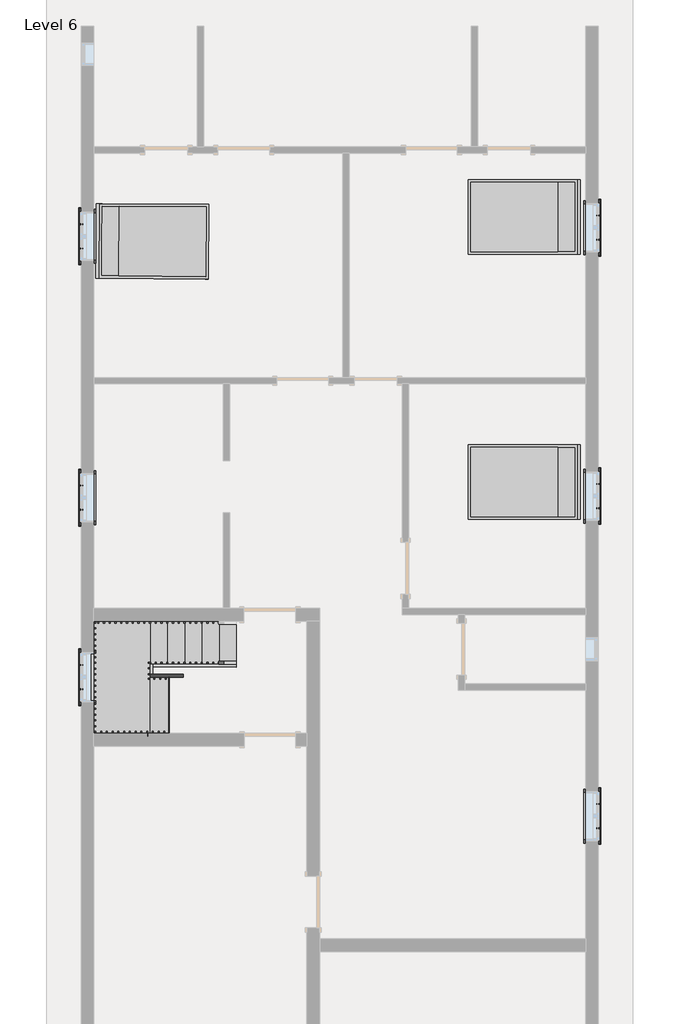
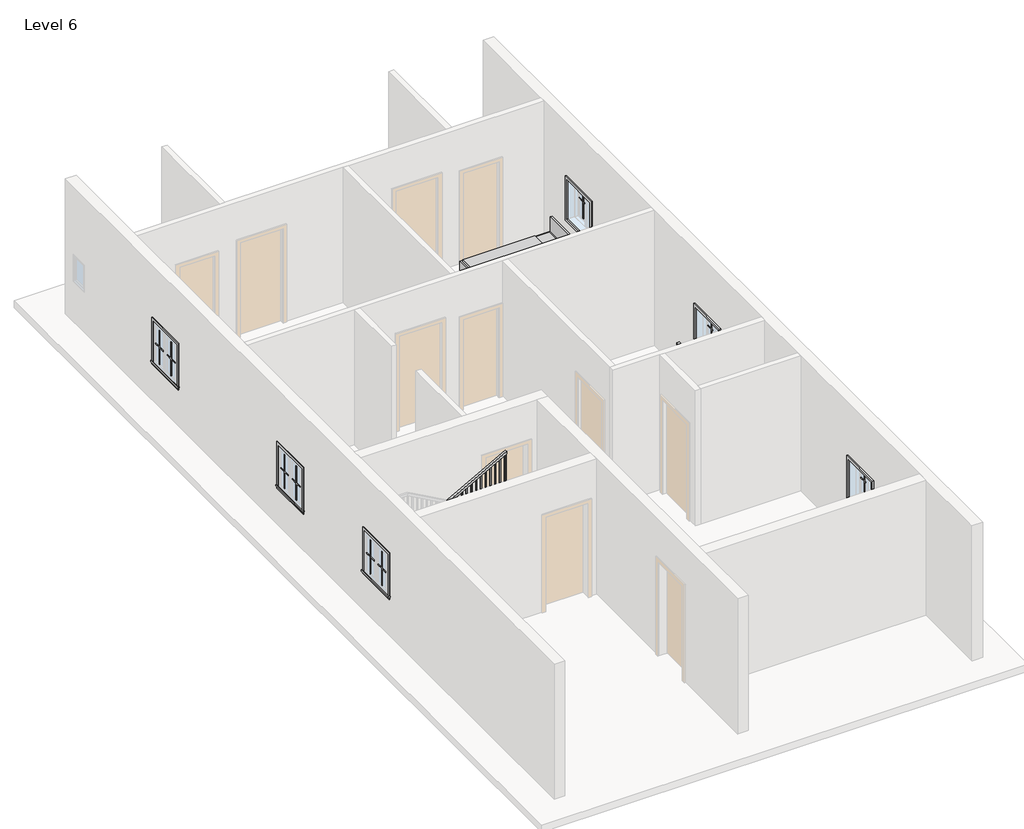
# One storey, part 3 of 3: 24 proxies, 6 members, 3 furniture elements, 1 railing, 1 stair flight.
"""IFC4 building model written with IfcOpenShell, lengths in millimetres."""

from ifc_helpers import new_model, si_unit, frame, origin, place, context, project, spatial, polyline, outline, extrude, faceted_brep, transform, mapped, element, save
from components import muntin_pattern_2x2_muntin_pattern_2x2_b3fe6957, muntin_pattern_2x2_muntin_pattern_2x2_3e0ecaf2, trim_window_exterior_flat_with_sill_41619996, trim_window_interior_flat_picture_frame_51c85655, bed_17739_bed_17739_15c61121, stair_flight_ed5f4c0f

model = new_model("IFC4")

# Units and contexts
model_context = context("Model", 3, world=origin())
ifc_project = project(units=[si_unit("LENGTHUNIT", "METRE", prefix="MILLI")], contexts=[model_context])

# Site, building, storey
site = spatial("IfcSite", under=ifc_project)
building = spatial("IfcBuilding", under=site)
storey = spatial("IfcBuildingStorey", under=building, Name="Level 6", Elevation=12801.6)

# Proxies
placement = place(None, origin())
muntin_pattern_2x2_muntin_pattern_2x2_shape = muntin_pattern_2x2_muntin_pattern_2x2_b3fe6957(model_context)
element("IfcBuildingElementProxy", 1, Name="Muntin Pattern_2x2 : Muntin Pattern_2x2", ObjectType="Muntin Pattern_2x2 : Muntin Pattern_2x2", at=placement, inside=storey, context=model_context, shape_type="MappedRepresentation", body=[
    mapped(muntin_pattern_2x2_muntin_pattern_2x2_shape, transform((3307.2334916, 6850.4197267, 13785.85), x_axis=(0.0, -1.0, 0.0), y_axis=(1.0, 0.0, 0.0), z_axis=(0.0, 0.0, 1.0))),
])
element("IfcBuildingElementProxy", 2, Name="Muntin Pattern_2x2 : Muntin Pattern_2x2", ObjectType="Muntin Pattern_2x2 : Muntin Pattern_2x2", at=placement, inside=storey, context=model_context, shape_type="MappedRepresentation", body=[
    mapped(muntin_pattern_2x2_muntin_pattern_2x2_shape, transform((3307.2334916, 2106.9697267, 13785.85), x_axis=(0.0, -1.0, 0.0), y_axis=(1.0, 0.0, 0.0), z_axis=(0.0, 0.0, 1.0))),
])
element("IfcBuildingElementProxy", 3, Name="Muntin Pattern_2x2 : Muntin Pattern_2x2", ObjectType="Muntin Pattern_2x2 : Muntin Pattern_2x2", at=placement, inside=storey, context=model_context, shape_type="MappedRepresentation", body=[
    mapped(muntin_pattern_2x2_muntin_pattern_2x2_shape, transform((-5817.7165084, 6269.3947267, 13785.85), x_axis=(0.0, 1.0, 0.0), y_axis=(-1.0, 0.0, 0.0), z_axis=(0.0, 0.0, 1.0))),
])
element("IfcBuildingElementProxy", 4, Name="Muntin Pattern_2x2 : Muntin Pattern_2x2", ObjectType="Muntin Pattern_2x2 : Muntin Pattern_2x2", at=placement, inside=storey, context=model_context, shape_type="MappedRepresentation", body=[
    mapped(muntin_pattern_2x2_muntin_pattern_2x2_shape, transform((-5817.7165084, 1649.7697267, 13785.85), x_axis=(0.0, 1.0, 0.0), y_axis=(-1.0, 0.0, 0.0), z_axis=(0.0, 0.0, 1.0))),
])
element("IfcBuildingElementProxy", 5, Name="Muntin Pattern_2x2 : Muntin Pattern_2x2", ObjectType="Muntin Pattern_2x2 : Muntin Pattern_2x2", at=placement, inside=storey, context=model_context, shape_type="MappedRepresentation", body=[
    mapped(muntin_pattern_2x2_muntin_pattern_2x2_shape, transform((3307.2334916, -3547.7052733, 13785.85), x_axis=(0.0, -1.0, 0.0), y_axis=(1.0, 0.0, 0.0), z_axis=(0.0, 0.0, 1.0))),
])
element("IfcBuildingElementProxy", 6, Name="Muntin Pattern_2x2 : Muntin Pattern_2x2", ObjectType="Muntin Pattern_2x2 : Muntin Pattern_2x2", at=placement, inside=storey, context=model_context, shape_type="MappedRepresentation", body=[
    mapped(muntin_pattern_2x2_muntin_pattern_2x2_shape, transform((-5817.7165084, -1522.0552733, 13785.85), x_axis=(0.0, 1.0, 0.0), y_axis=(-1.0, 0.0, 0.0), z_axis=(0.0, 0.0, 1.0))),
])
muntin_pattern_2x2_muntin_pattern_2x2_2_shape = muntin_pattern_2x2_muntin_pattern_2x2_3e0ecaf2(model_context)
element("IfcBuildingElementProxy", 7, Name="Muntin Pattern_2x2 : Muntin Pattern_2x2", ObjectType="Muntin Pattern_2x2 : Muntin Pattern_2x2", at=placement, inside=storey, context=model_context, shape_type="MappedRepresentation", body=[
    mapped(muntin_pattern_2x2_muntin_pattern_2x2_2_shape, transform((3307.2334916, 6421.7947267, 13785.85), x_axis=(0.0, 1.0, 0.0), y_axis=(-1.0, 0.0, 0.0), z_axis=(0.0, 0.0, 1.0))),
])
element("IfcBuildingElementProxy", 8, Name="Muntin Pattern_2x2 : Muntin Pattern_2x2", ObjectType="Muntin Pattern_2x2 : Muntin Pattern_2x2", at=placement, inside=storey, context=model_context, shape_type="MappedRepresentation", body=[
    mapped(muntin_pattern_2x2_muntin_pattern_2x2_2_shape, transform((3307.2334916, 1678.3447267, 13785.85), x_axis=(0.0, 1.0, 0.0), y_axis=(-1.0, 0.0, 0.0), z_axis=(0.0, 0.0, 1.0))),
])
element("IfcBuildingElementProxy", 9, Name="Muntin Pattern_2x2 : Muntin Pattern_2x2", ObjectType="Muntin Pattern_2x2 : Muntin Pattern_2x2", at=placement, inside=storey, context=model_context, shape_type="MappedRepresentation", body=[
    mapped(muntin_pattern_2x2_muntin_pattern_2x2_2_shape, transform((-5817.7165084, 6698.0197267, 13785.85), x_axis=(0.0, -1.0, 0.0), y_axis=(1.0, 0.0, 0.0), z_axis=(0.0, 0.0, 1.0))),
])
element("IfcBuildingElementProxy", 10, Name="Muntin Pattern_2x2 : Muntin Pattern_2x2", ObjectType="Muntin Pattern_2x2 : Muntin Pattern_2x2", at=placement, inside=storey, context=model_context, shape_type="MappedRepresentation", body=[
    mapped(muntin_pattern_2x2_muntin_pattern_2x2_2_shape, transform((-5817.7165084, 2078.3947267, 13785.85), x_axis=(0.0, -1.0, 0.0), y_axis=(1.0, 0.0, 0.0), z_axis=(0.0, 0.0, 1.0))),
])
element("IfcBuildingElementProxy", 11, Name="Muntin Pattern_2x2 : Muntin Pattern_2x2", ObjectType="Muntin Pattern_2x2 : Muntin Pattern_2x2", at=placement, inside=storey, context=model_context, shape_type="MappedRepresentation", body=[
    mapped(muntin_pattern_2x2_muntin_pattern_2x2_2_shape, transform((3307.2334916, -3976.3302733, 13785.85), x_axis=(0.0, 1.0, 0.0), y_axis=(-1.0, 0.0, 0.0), z_axis=(0.0, 0.0, 1.0))),
])
element("IfcBuildingElementProxy", 12, Name="Muntin Pattern_2x2 : Muntin Pattern_2x2", ObjectType="Muntin Pattern_2x2 : Muntin Pattern_2x2", at=placement, inside=storey, context=model_context, shape_type="MappedRepresentation", body=[
    mapped(muntin_pattern_2x2_muntin_pattern_2x2_2_shape, transform((-5817.7165084, -1093.4302733, 13785.85), x_axis=(0.0, -1.0, 0.0), y_axis=(1.0, 0.0, 0.0), z_axis=(0.0, 0.0, 1.0))),
])
trim_window_exterior_flat_with_sill_shape = trim_window_exterior_flat_with_sill_41619996(model_context)
element("IfcBuildingElementProxy", 13, Name="Trim-Window-Exterior-Flat : with Sill", ObjectType="Trim-Window-Exterior-Flat : with Sill", at=placement, inside=storey, context=model_context, shape_type="MappedRepresentation", body=[
    mapped(trim_window_exterior_flat_with_sill_shape, transform((3316.7584916, 6636.1072267, 14630.4), x_axis=(0.0, 1.0, 0.0), y_axis=(0.0, 0.0, 1.0), z_axis=(1.0, 0.0, 0.0))),
])
element("IfcBuildingElementProxy", 14, Name="Trim-Window-Exterior-Flat : with Sill", ObjectType="Trim-Window-Exterior-Flat : with Sill", at=placement, inside=storey, context=model_context, shape_type="MappedRepresentation", body=[
    mapped(trim_window_exterior_flat_with_sill_shape, transform((3316.7584916, 1892.6572267, 14630.4), x_axis=(0.0, 1.0, 0.0), y_axis=(0.0, 0.0, 1.0), z_axis=(1.0, 0.0, 0.0))),
])
element("IfcBuildingElementProxy", 15, Name="Trim-Window-Exterior-Flat : with Sill", ObjectType="Trim-Window-Exterior-Flat : with Sill", at=placement, inside=storey, context=model_context, shape_type="MappedRepresentation", body=[
    mapped(trim_window_exterior_flat_with_sill_shape, transform((-5827.2415084, 6483.7072267, 14630.4), x_axis=(0.0, -1.0, 0.0), y_axis=(0.0, 0.0, 1.0), z_axis=(-1.0, 0.0, 0.0))),
])
element("IfcBuildingElementProxy", 16, Name="Trim-Window-Exterior-Flat : with Sill", ObjectType="Trim-Window-Exterior-Flat : with Sill", at=placement, inside=storey, context=model_context, shape_type="MappedRepresentation", body=[
    mapped(trim_window_exterior_flat_with_sill_shape, transform((-5827.2415084, 1864.0822267, 14630.4), x_axis=(0.0, -1.0, 0.0), y_axis=(0.0, 0.0, 1.0), z_axis=(-1.0, 0.0, 0.0))),
])
element("IfcBuildingElementProxy", 17, Name="Trim-Window-Exterior-Flat : with Sill", ObjectType="Trim-Window-Exterior-Flat : with Sill", at=placement, inside=storey, context=model_context, shape_type="MappedRepresentation", body=[
    mapped(trim_window_exterior_flat_with_sill_shape, transform((3316.7584916, -3762.0177733, 14630.4), x_axis=(0.0, 1.0, 0.0), y_axis=(0.0, 0.0, 1.0), z_axis=(1.0, 0.0, 0.0))),
])
element("IfcBuildingElementProxy", 18, Name="Trim-Window-Exterior-Flat : with Sill", ObjectType="Trim-Window-Exterior-Flat : with Sill", at=placement, inside=storey, context=model_context, shape_type="MappedRepresentation", body=[
    mapped(trim_window_exterior_flat_with_sill_shape, transform((-5827.2415084, -1307.7427733, 14630.4), x_axis=(0.0, -1.0, 0.0), y_axis=(0.0, 0.0, 1.0), z_axis=(-1.0, 0.0, 0.0))),
])
trim_window_interior_flat_picture_frame_shape = trim_window_interior_flat_picture_frame_51c85655(model_context)
element("IfcBuildingElementProxy", 19, Name="Trim-Window-Interior-Flat : Picture Frame", ObjectType="Trim-Window-Interior-Flat : Picture Frame", at=placement, inside=storey, context=model_context, shape_type="MappedRepresentation", body=[
    mapped(trim_window_interior_flat_picture_frame_shape, transform((3088.1584916, 6636.1072267, 14630.4), x_axis=(0.0, -1.0, 0.0), y_axis=(0.0, 0.0, 1.0), z_axis=(-1.0, 0.0, 0.0))),
])
element("IfcBuildingElementProxy", 20, Name="Trim-Window-Interior-Flat : Picture Frame", ObjectType="Trim-Window-Interior-Flat : Picture Frame", at=placement, inside=storey, context=model_context, shape_type="MappedRepresentation", body=[
    mapped(trim_window_interior_flat_picture_frame_shape, transform((3088.1584916, 1892.6572267, 14630.4), x_axis=(0.0, -1.0, 0.0), y_axis=(0.0, 0.0, 1.0), z_axis=(-1.0, 0.0, 0.0))),
])
element("IfcBuildingElementProxy", 21, Name="Trim-Window-Interior-Flat : Picture Frame", ObjectType="Trim-Window-Interior-Flat : Picture Frame", at=placement, inside=storey, context=model_context, shape_type="MappedRepresentation", body=[
    mapped(trim_window_interior_flat_picture_frame_shape, transform((-5598.6415084, 6483.7072267, 14630.4), x_axis=(0.0, 1.0, 0.0), y_axis=(0.0, 0.0, 1.0), z_axis=(1.0, 0.0, 0.0))),
])
element("IfcBuildingElementProxy", 22, Name="Trim-Window-Interior-Flat : Picture Frame", ObjectType="Trim-Window-Interior-Flat : Picture Frame", at=placement, inside=storey, context=model_context, shape_type="MappedRepresentation", body=[
    mapped(trim_window_interior_flat_picture_frame_shape, transform((-5598.6415084, 1864.0822267, 14630.4), x_axis=(0.0, 1.0, 0.0), y_axis=(0.0, 0.0, 1.0), z_axis=(1.0, 0.0, 0.0))),
])
element("IfcBuildingElementProxy", 23, Name="Trim-Window-Interior-Flat : Picture Frame", ObjectType="Trim-Window-Interior-Flat : Picture Frame", at=placement, inside=storey, context=model_context, shape_type="MappedRepresentation", body=[
    mapped(trim_window_interior_flat_picture_frame_shape, transform((3088.1584916, -3762.0177733, 14630.4), x_axis=(0.0, -1.0, 0.0), y_axis=(0.0, 0.0, 1.0), z_axis=(-1.0, 0.0, 0.0))),
])
element("IfcBuildingElementProxy", 24, Name="Trim-Window-Interior-Flat : Picture Frame", ObjectType="Trim-Window-Interior-Flat : Picture Frame", at=placement, inside=storey, context=model_context, shape_type="MappedRepresentation", body=[
    mapped(trim_window_interior_flat_picture_frame_shape, transform((-5598.6415084, -1307.7427733, 14630.4), x_axis=(0.0, 1.0, 0.0), y_axis=(0.0, 0.0, 1.0), z_axis=(1.0, 0.0, 0.0))),
])

# Furniture
bed_17739_bed_17739_shape = bed_17739_bed_17739_15c61121(model_context)
element("IfcFurniture", 25, ObjectType="Bed_17739 : Bed_17739", at=placement, inside=storey, context=model_context, shape_type="MappedRepresentation", body=[
    mapped(bed_17739_bed_17739_shape, transform((-4543.6279345, 6394.2844586, 12801.6), x_axis=(0.007593038844487308, 0.9999711724650396, 0.0), y_axis=(-0.9999711724650396, 0.007593038844487308, 0.0), z_axis=(0.0, 0.0, 1.0))),
])
element("IfcFurniture", 26, ObjectType="Bed_17739 : Bed_17739", at=placement, inside=storey, context=model_context, shape_type="MappedRepresentation", body=[
    mapped(bed_17739_bed_17739_shape, transform((1983.2584916, 6826.6072267, 12801.6), x_axis=(0.0, -1.0, 0.0), y_axis=(1.0, 0.0, 0.0), z_axis=(0.0, 0.0, 1.0))),
])
element("IfcFurniture", 27, ObjectType="Bed_17739 : Bed_17739", at=placement, inside=storey, context=model_context, shape_type="MappedRepresentation", body=[
    mapped(bed_17739_bed_17739_shape, transform((1983.2584916, 2140.3072267, 12801.6), x_axis=(0.0, -1.0, 0.0), y_axis=(1.0, 0.0, 0.0), z_axis=(0.0, 0.0, 1.0))),
])

# Members
element("IfcMember", 28, ObjectType="Stringer - 2\" Width", at=placement, inside=storey, context=model_context, shape_type="SweptSolid", body=[
    extrude(outline(polyline([(12801.6, -3084.0415084), (13009.1983948, -3084.0415084), (13827.6428392, -4557.2415084), (13478.9641651, -4557.2415084), (12801.6, -3337.9860112), (12801.6, -3084.0415084)])), frame((0.0, -1127.4758739, 0.0), z_axis=(0.0, 1.0, 0.0), x_axis=(0.0, 0.0, 1.0)), (0.0, 0.0, 1.0), 50.8),
])
element("IfcMember", 29, ObjectType="Stringer - 2\" Width", at=placement, inside=storey, context=model_context, shape_type="SweptSolid", body=[
    extrude(outline(polyline([(-4608.0415084, -1076.6758739), (-4557.2415084, -1076.6758739), (-4557.2415084, -1256.9427733), (-4608.0415084, -1256.9427733), (-4608.0415084, -1076.6758739)])), frame((0.0, 0.0, 13589.0), z_axis=(0.0, 0.0, 1.0), x_axis=(1.0, 0.0, 0.0)), (0.0, 0.0, 1.0), 304.8),
])
element("IfcMember", 30, ObjectType="Stringer - 2\" Width", at=placement, inside=storey, context=model_context, shape_type="SweptSolid", body=[
    extrude(outline(polyline([(14025.1983948, -4608.0415084), (13676.5197207, -4608.0415084), (14523.1863873, -3084.0415084), (14871.8650614, -3084.0415084), (14025.1983948, -4608.0415084)])), frame((0.0, -1307.7427733, 0.0), z_axis=(0.0, 1.0, 0.0), x_axis=(0.0, 0.0, 1.0)), (0.0, 0.0, 1.0), 50.8),
])
element("IfcMember", 31, ObjectType="Stringer - 2\" Width", at=placement, inside=storey, context=model_context, shape_type="SweptSolid", body=[
    extrude(outline(polyline([(12801.6, -3084.0415084), (13009.1983948, -3084.0415084), (13893.8, -4676.3243978), (13893.8, -5303.9460112), (12801.6, -3337.9860112), (12801.6, -3084.0415084)])), frame((0.0, -317.1427733, 0.0), z_axis=(0.0, 1.0, 0.0), x_axis=(0.0, 0.0, 1.0)), (0.0, 0.0, 1.0), 50.8),
])
element("IfcMember", 32, ObjectType="Stringer - 2\" Width", at=placement, inside=storey, context=model_context, shape_type="SweptSolid", body=[
    extrude(outline(polyline([(-5649.4415084, -266.3427733), (-5598.6415084, -266.3427733), (-5598.6415084, -2298.3427733), (-5649.4415084, -2298.3427733), (-5649.4415084, -266.3427733)])), frame((0.0, 0.0, 13589.0), z_axis=(0.0, 0.0, 1.0), x_axis=(1.0, 0.0, 0.0)), (0.0, 0.0, 1.0), 304.8),
])
element("IfcMember", 33, ObjectType="Stringer - 2\" Width", at=placement, inside=storey, context=model_context, shape_type="SweptSolid", body=[
    extrude(outline(polyline([(13589.0, -4765.5770056), (14523.1863873, -3084.0415084), (14871.8650614, -3084.0415084), (13589.0, -5393.198619), (13589.0, -4765.5770056)])), frame((0.0, -2349.1427733, 0.0), z_axis=(0.0, 1.0, 0.0), x_axis=(0.0, 0.0, 1.0)), (0.0, 0.0, 1.0), 50.8),
])

# Railing
element("IfcRailing", 34, ObjectType="Handrail - Rectangular", at=placement, inside=storey, context=model_context, shape_type="SolidModel", body=[
    faceted_brep([(-3084.0415084, -1076.6758739, 13885.3333333), (-3084.0415084, -1076.6758739, 13827.220221), (-3084.0415084, -1025.8758739, 13827.220221), (-3084.0415084, -1025.8758739, 13885.3333333), (-4531.8415084, -1076.6758739, 14689.6666667), (-4582.6415084, -1076.6758739, 14659.7757765), (-4582.6415084, -1025.8758739, 14659.7757765), (-4531.8415084, -1025.8758739, 14689.6666667), (-4531.8415084, -1076.6758739, 14732.0), (-4582.6415084, -1076.6758739, 14681.2), (-4582.6415084, -1025.8758739, 14681.2), (-4531.8415084, -1025.8758739, 14732.0), (-4608.0415084, -1076.6758739, 14732.0), (-4608.0415084, -1076.6758739, 14681.2), (-4658.8415084, -1025.8758739, 14681.2), (-4658.8415084, -1025.8758739, 14732.0), (-4608.0415084, -1152.8758739, 14732.0), (-4608.0415084, -1152.8758739, 14681.2), (-4658.8415084, -1152.8758739, 14681.2), (-4658.8415084, -1152.8758739, 14732.0), (-4608.0415084, -1231.5427733, 14732.0), (-4608.0415084, -1282.3427733, 14681.2), (-4658.8415084, -1282.3427733, 14681.2), (-4658.8415084, -1231.5427733, 14732.0), (-4608.0415084, -1231.5427733, 14943.6666667), (-4608.0415084, -1282.3427733, 14892.8666667), (-4658.8415084, -1282.3427733, 14892.8666667), (-4658.8415084, -1231.5427733, 14943.6666667), (-4608.0415084, -1307.7427733, 14943.6666667), (-4608.0415084, -1307.7427733, 14892.8666667), (-4658.8415084, -1358.5427733, 14892.8666667), (-4658.8415084, -1358.5427733, 14943.6666667), (-4531.8415084, -1307.7427733, 14943.6666667), (-4518.6779062, -1307.7427733, 14892.8666667), (-4518.6779062, -1358.5427733, 14892.8666667), (-4531.8415084, -1358.5427733, 14943.6666667), (-3084.0415084, -1307.7427733, 15748.0), (-3084.0415084, -1358.5427733, 15748.0), (-3084.0415084, -1358.5427733, 15689.8868876), (-3084.0415084, -1307.7427733, 15689.8868876)], [[[0, 1, 2, 3]], [[1, 0, 4, 5]], [[2, 1, 5, 6]], [[3, 2, 6, 7]], [[0, 3, 7, 4]], [[5, 4, 8, 9]], [[6, 5, 9, 10]], [[7, 6, 10, 11]], [[4, 7, 11, 8]], [[9, 8, 12, 13]], [[10, 9, 13, 14]], [[11, 10, 14, 15]], [[8, 11, 15, 12]], [[13, 12, 16, 17]], [[14, 13, 17, 18]], [[15, 14, 18, 19]], [[12, 15, 19, 16]], [[17, 16, 20, 21]], [[18, 17, 21, 22]], [[19, 18, 22, 23]], [[16, 19, 23, 20]], [[21, 20, 24, 25]], [[22, 21, 25, 26]], [[23, 22, 26, 27]], [[20, 23, 27, 24]], [[25, 24, 28, 29]], [[26, 25, 29, 30]], [[27, 26, 30, 31]], [[24, 27, 31, 28]], [[29, 28, 32, 33]], [[30, 29, 33, 34]], [[31, 30, 34, 35]], [[28, 31, 35, 32]], [[36, 37, 38, 39]], [[33, 32, 36, 39]], [[34, 33, 39, 38]], [[35, 34, 38, 37]], [[32, 35, 37, 36]]]),
    extrude(outline(polyline([(15670.4841099, -3118.9665084), (14664.2666667, -3118.9665084), (14664.2666667, -3099.9165084), (15681.0674432, -3099.9165084), (15670.4841099, -3118.9665084)])), frame((0.0, -1342.6677733, 0.0), z_axis=(0.0, 1.0, 0.0), x_axis=(0.0, 0.0, 1.0)), (0.0, 0.0, 1.0), 19.05),
    extrude(outline(polyline([(15614.0396654, -3220.5665084), (14664.2666667, -3220.5665084), (14664.2666667, -3201.5165084), (15624.6229988, -3201.5165084), (15614.0396654, -3220.5665084)])), frame((0.0, -1342.6677733, 0.0), z_axis=(0.0, 1.0, 0.0), x_axis=(0.0, 0.0, 1.0)), (0.0, 0.0, 1.0), 19.05),
    extrude(outline(polyline([(15557.595221, -3322.1665084), (14664.2666667, -3322.1665084), (14664.2666667, -3303.1165084), (15568.1785543, -3303.1165084), (15557.595221, -3322.1665084)])), frame((0.0, -1342.6677733, 0.0), z_axis=(0.0, 1.0, 0.0), x_axis=(0.0, 0.0, 1.0)), (0.0, 0.0, 1.0), 19.05),
    extrude(outline(polyline([(15501.1507765, -3423.7665084), (14494.9333333, -3423.7665084), (14494.9333333, -3404.7165084), (15511.7341099, -3404.7165084), (15501.1507765, -3423.7665084)])), frame((0.0, -1342.6677733, 0.0), z_axis=(0.0, 1.0, 0.0), x_axis=(0.0, 0.0, 1.0)), (0.0, 0.0, 1.0), 19.05),
    extrude(outline(polyline([(15444.7063321, -3525.3665084), (14494.9333333, -3525.3665084), (14494.9333333, -3506.3165084), (15455.2896654, -3506.3165084), (15444.7063321, -3525.3665084)])), frame((0.0, -1342.6677733, 0.0), z_axis=(0.0, 1.0, 0.0), x_axis=(0.0, 0.0, 1.0)), (0.0, 0.0, 1.0), 19.05),
    extrude(outline(polyline([(15388.2618876, -3626.9665084), (14494.9333333, -3626.9665084), (14494.9333333, -3607.9165084), (15398.845221, -3607.9165084), (15388.2618876, -3626.9665084)])), frame((0.0, -1342.6677733, 0.0), z_axis=(0.0, 1.0, 0.0), x_axis=(0.0, 0.0, 1.0)), (0.0, 0.0, 1.0), 19.05),
    extrude(outline(polyline([(15331.8174432, -3728.5665084), (14325.6, -3728.5665084), (14325.6, -3709.5165084), (15342.4007765, -3709.5165084), (15331.8174432, -3728.5665084)])), frame((0.0, -1342.6677733, 0.0), z_axis=(0.0, 1.0, 0.0), x_axis=(0.0, 0.0, 1.0)), (0.0, 0.0, 1.0), 19.05),
    extrude(outline(polyline([(15275.3729988, -3830.1665084), (14325.6, -3830.1665084), (14325.6, -3811.1165084), (15285.9563321, -3811.1165084), (15275.3729988, -3830.1665084)])), frame((0.0, -1342.6677733, 0.0), z_axis=(0.0, 1.0, 0.0), x_axis=(0.0, 0.0, 1.0)), (0.0, 0.0, 1.0), 19.05),
    extrude(outline(polyline([(15218.9285543, -3931.7665084), (14325.6, -3931.7665084), (14325.6, -3912.7165084), (15229.5118876, -3912.7165084), (15218.9285543, -3931.7665084)])), frame((0.0, -1342.6677733, 0.0), z_axis=(0.0, 1.0, 0.0), x_axis=(0.0, 0.0, 1.0)), (0.0, 0.0, 1.0), 19.05),
    extrude(outline(polyline([(15162.4841099, -4033.3665084), (14156.2666667, -4033.3665084), (14156.2666667, -4014.3165084), (15173.0674432, -4014.3165084), (15162.4841099, -4033.3665084)])), frame((0.0, -1342.6677733, 0.0), z_axis=(0.0, 1.0, 0.0), x_axis=(0.0, 0.0, 1.0)), (0.0, 0.0, 1.0), 19.05),
    extrude(outline(polyline([(15106.0396654, -4134.9665084), (14156.2666667, -4134.9665084), (14156.2666667, -4115.9165084), (15116.6229988, -4115.9165084), (15106.0396654, -4134.9665084)])), frame((0.0, -1342.6677733, 0.0), z_axis=(0.0, 1.0, 0.0), x_axis=(0.0, 0.0, 1.0)), (0.0, 0.0, 1.0), 19.05),
    extrude(outline(polyline([(15049.595221, -4236.5665084), (14156.2666667, -4236.5665084), (14156.2666667, -4217.5165084), (15060.1785543, -4217.5165084), (15049.595221, -4236.5665084)])), frame((0.0, -1342.6677733, 0.0), z_axis=(0.0, 1.0, 0.0), x_axis=(0.0, 0.0, 1.0)), (0.0, 0.0, 1.0), 19.05),
    extrude(outline(polyline([(14993.1507765, -4338.1665084), (13986.9333333, -4338.1665084), (13986.9333333, -4319.1165084), (15003.7341099, -4319.1165084), (14993.1507765, -4338.1665084)])), frame((0.0, -1342.6677733, 0.0), z_axis=(0.0, 1.0, 0.0), x_axis=(0.0, 0.0, 1.0)), (0.0, 0.0, 1.0), 19.05),
    extrude(outline(polyline([(14936.7063321, -4439.7665084), (13986.9333333, -4439.7665084), (13986.9333333, -4420.7165084), (14947.2896654, -4420.7165084), (14936.7063321, -4439.7665084)])), frame((0.0, -1342.6677733, 0.0), z_axis=(0.0, 1.0, 0.0), x_axis=(0.0, 0.0, 1.0)), (0.0, 0.0, 1.0), 19.05),
    extrude(outline(polyline([(14880.2618876, -4541.3665084), (13986.9333333, -4541.3665084), (13986.9333333, -4522.3165084), (14890.845221, -4522.3165084), (14880.2618876, -4541.3665084)])), frame((0.0, -1342.6677733, 0.0), z_axis=(0.0, 1.0, 0.0), x_axis=(0.0, 0.0, 1.0)), (0.0, 0.0, 1.0), 19.05),
    extrude(outline(polyline([(-4623.9165084, -1244.9508739), (-4623.9165084, -1264.0008739), (-4642.9665084, -1264.0008739), (-4642.9665084, -1244.9508739), (-4623.9165084, -1244.9508739)])), frame((0.0, 0.0, 13817.6), z_axis=(0.0, 0.0, 1.0), x_axis=(1.0, 0.0, 0.0)), (0.0, 0.0, 1.0), 1075.2666667),
    extrude(outline(polyline([(-4623.9165084, -1143.3508739), (-4623.9165084, -1162.4008739), (-4642.9665084, -1162.4008739), (-4642.9665084, -1143.3508739), (-4623.9165084, -1143.3508739)])), frame((0.0, 0.0, 13817.6), z_axis=(0.0, 0.0, 1.0), x_axis=(1.0, 0.0, 0.0)), (0.0, 0.0, 1.0), 863.6),
    extrude(outline(polyline([(-4598.5165084, -1060.8008739), (-4617.5665084, -1060.8008739), (-4617.5665084, -1041.7508739), (-4598.5165084, -1041.7508739), (-4598.5165084, -1060.8008739)])), frame((0.0, 0.0, 13817.6), z_axis=(0.0, 0.0, 1.0), x_axis=(1.0, 0.0, 0.0)), (0.0, 0.0, 1.0), 863.6),
    extrude(outline(polyline([(14622.7341099, -4515.9665084), (13648.2666667, -4515.9665084), (13648.2666667, -4496.9165084), (14612.1507765, -4496.9165084), (14622.7341099, -4515.9665084)])), frame((0.0, -1060.8008739, 0.0), z_axis=(0.0, 1.0, 0.0), x_axis=(0.0, 0.0, 1.0)), (0.0, 0.0, 1.0), 19.05),
    extrude(outline(polyline([(14566.2896654, -4414.3665084), (13648.2666667, -4414.3665084), (13648.2666667, -4395.3165084), (14555.7063321, -4395.3165084), (14566.2896654, -4414.3665084)])), frame((0.0, -1060.8008739, 0.0), z_axis=(0.0, 1.0, 0.0), x_axis=(0.0, 0.0, 1.0)), (0.0, 0.0, 1.0), 19.05),
    extrude(outline(polyline([(14509.845221, -4312.7665084), (13648.2666667, -4312.7665084), (13648.2666667, -4293.7165084), (14499.2618876, -4293.7165084), (14509.845221, -4312.7665084)])), frame((0.0, -1060.8008739, 0.0), z_axis=(0.0, 1.0, 0.0), x_axis=(0.0, 0.0, 1.0)), (0.0, 0.0, 1.0), 19.05),
    extrude(outline(polyline([(14453.4007765, -4211.1665084), (13478.9333333, -4211.1665084), (13478.9333333, -4192.1165084), (14442.8174432, -4192.1165084), (14453.4007765, -4211.1665084)])), frame((0.0, -1060.8008739, 0.0), z_axis=(0.0, 1.0, 0.0), x_axis=(0.0, 0.0, 1.0)), (0.0, 0.0, 1.0), 19.05),
    extrude(outline(polyline([(14396.9563321, -4109.5665084), (13478.9333333, -4109.5665084), (13478.9333333, -4090.5165084), (14386.3729988, -4090.5165084), (14396.9563321, -4109.5665084)])), frame((0.0, -1060.8008739, 0.0), z_axis=(0.0, 1.0, 0.0), x_axis=(0.0, 0.0, 1.0)), (0.0, 0.0, 1.0), 19.05),
    extrude(outline(polyline([(14340.5118876, -4007.9665084), (13478.9333333, -4007.9665084), (13478.9333333, -3988.9165084), (14329.9285543, -3988.9165084), (14340.5118876, -4007.9665084)])), frame((0.0, -1060.8008739, 0.0), z_axis=(0.0, 1.0, 0.0), x_axis=(0.0, 0.0, 1.0)), (0.0, 0.0, 1.0), 19.05),
    extrude(outline(polyline([(14284.0674432, -3906.3665084), (13309.6, -3906.3665084), (13309.6, -3887.3165084), (14273.4841099, -3887.3165084), (14284.0674432, -3906.3665084)])), frame((0.0, -1060.8008739, 0.0), z_axis=(0.0, 1.0, 0.0), x_axis=(0.0, 0.0, 1.0)), (0.0, 0.0, 1.0), 19.05),
    extrude(outline(polyline([(14227.6229988, -3804.7665084), (13309.6, -3804.7665084), (13309.6, -3785.7165084), (14217.0396654, -3785.7165084), (14227.6229988, -3804.7665084)])), frame((0.0, -1060.8008739, 0.0), z_axis=(0.0, 1.0, 0.0), x_axis=(0.0, 0.0, 1.0)), (0.0, 0.0, 1.0), 19.05),
    extrude(outline(polyline([(14171.1785543, -3703.1665084), (13309.6, -3703.1665084), (13309.6, -3684.1165084), (14160.595221, -3684.1165084), (14171.1785543, -3703.1665084)])), frame((0.0, -1060.8008739, 0.0), z_axis=(0.0, 1.0, 0.0), x_axis=(0.0, 0.0, 1.0)), (0.0, 0.0, 1.0), 19.05),
    extrude(outline(polyline([(14114.7341099, -3601.5665084), (13140.2666667, -3601.5665084), (13140.2666667, -3582.5165084), (14104.1507765, -3582.5165084), (14114.7341099, -3601.5665084)])), frame((0.0, -1060.8008739, 0.0), z_axis=(0.0, 1.0, 0.0), x_axis=(0.0, 0.0, 1.0)), (0.0, 0.0, 1.0), 19.05),
    extrude(outline(polyline([(14058.2896654, -3499.9665084), (13140.2666667, -3499.9665084), (13140.2666667, -3480.9165084), (14047.7063321, -3480.9165084), (14058.2896654, -3499.9665084)])), frame((0.0, -1060.8008739, 0.0), z_axis=(0.0, 1.0, 0.0), x_axis=(0.0, 0.0, 1.0)), (0.0, 0.0, 1.0), 19.05),
    extrude(outline(polyline([(14001.845221, -3398.3665084), (13140.2666667, -3398.3665084), (13140.2666667, -3379.3165084), (13991.2618876, -3379.3165084), (14001.845221, -3398.3665084)])), frame((0.0, -1060.8008739, 0.0), z_axis=(0.0, 1.0, 0.0), x_axis=(0.0, 0.0, 1.0)), (0.0, 0.0, 1.0), 19.05),
    extrude(outline(polyline([(13945.4007765, -3296.7665084), (12970.9333333, -3296.7665084), (12970.9333333, -3277.7165084), (13934.8174432, -3277.7165084), (13945.4007765, -3296.7665084)])), frame((0.0, -1060.8008739, 0.0), z_axis=(0.0, 1.0, 0.0), x_axis=(0.0, 0.0, 1.0)), (0.0, 0.0, 1.0), 19.05),
    extrude(outline(polyline([(13888.9563321, -3195.1665084), (12970.9333333, -3195.1665084), (12970.9333333, -3176.1165084), (13878.3729988, -3176.1165084), (13888.9563321, -3195.1665084)])), frame((0.0, -1060.8008739, 0.0), z_axis=(0.0, 1.0, 0.0), x_axis=(0.0, 0.0, 1.0)), (0.0, 0.0, 1.0), 19.05),
    extrude(outline(polyline([(-4623.9165084, -1323.6177733), (-4623.9165084, -1342.6677733), (-4642.9665084, -1342.6677733), (-4642.9665084, -1323.6177733), (-4623.9165084, -1323.6177733)])), frame((0.0, 0.0, 13817.6), z_axis=(0.0, 0.0, 1.0), x_axis=(1.0, 0.0, 0.0)), (0.0, 0.0, 1.0), 1075.2666667),
    extrude(outline(polyline([(-4623.9165084, -1060.8008739), (-4642.9665084, -1060.8008739), (-4642.9665084, -1041.7508739), (-4623.9165084, -1041.7508739), (-4623.9165084, -1060.8008739)])), frame((0.0, 0.0, 13817.6), z_axis=(0.0, 0.0, 1.0), x_axis=(1.0, 0.0, 0.0)), (0.0, 0.0, 1.0), 863.6),
    extrude(outline(polyline([(15679.3035543, -3103.0915084), (14664.2666667, -3103.0915084), (14664.2666667, -3084.0415084), (15689.8868876, -3084.0415084), (15679.3035543, -3103.0915084)])), frame((0.0, -1342.6677733, 0.0), z_axis=(0.0, 1.0, 0.0), x_axis=(0.0, 0.0, 1.0)), (0.0, 0.0, 1.0), 19.05),
    extrude(outline(polyline([(13837.8035543, -3103.0915084), (12970.9333333, -3103.0915084), (12970.9333333, -3084.0415084), (13827.220221, -3084.0415084), (13837.8035543, -3103.0915084)])), frame((0.0, -1060.8008739, 0.0), z_axis=(0.0, 1.0, 0.0), x_axis=(0.0, 0.0, 1.0)), (0.0, 0.0, 1.0), 19.05),
])

# Stair flight
stair_flight_shape = stair_flight_ed5f4c0f(model_context)
element("IfcStairFlight", 35, ObjectType="2\" Tread 1\" Nosing 1/4\" Riser", at=placement, inside=storey, context=model_context, shape_type="MappedRepresentation", body=[
    mapped(stair_flight_shape, transform((0.0, 0.0, 0.0), x_axis=(1.0, 0.0, 0.0), y_axis=(0.0, 1.0, 0.0), z_axis=(0.0, 0.0, 1.0))),
])

save(model, "model.ifc")

# Revit data of these elements
# Type "Muntin Pattern_2x2 : Muntin Pattern_2x2"
#   Width [instance default] = 4' - 0"
#   Thickness = 0' - 0 1/2"
#   Height [instance default] = 4' - 0"
#   Distance = 0' - 0 3/4"
#   Interior Material [instance default] = none
#   Exterior Material [instance default] = none
#   Default Elevation = 0
# Type "Trim-Window-Exterior-Flat : with Sill"
#   Trim Width = 0' - 2 1/4"
#   Trim Thickness_Picture Frame = 0' - 1 1/4"
#   Trim Thickness_with Sill = 0' - 0 3/4"
#   Sill Thickness = 0' - 1 1/4"
#   Opening Width [instance default] = 2' - 0"
#   Opening Height [instance default] = 3' - 0"
#   Default Elevation = 4' - 0"
#   Sill = yes
#   Picture Frame = no
#   Trim Material [instance default] = none
# Type "Trim-Window-Interior-Flat : Picture Frame"
#   Trim Thickness_Picture Frame = 0' - 1 1/4"
#   Trim Width = 0' - 2 1/4"
#   Trim Thickness_with Sill = 0' - 0 3/4"
#   Sill Thickness = 0' - 1 1/4"
#   Opening Width [instance default] = 2' - 0"
#   Opening Height [instance default] = 3' - 0"
#   Default Elevation = 4' - 0"
#   Sill = no
#   Picture Frame = yes
#   Trim Material [instance default] = none
# Type "Bed_17739 : Bed_17739"
#   Default Elevation = 0
# Type "Handrail - Rectangular"
#   Assembly Code = "C2010400"
#   built-in parameter 1008612 = 0.0416667 (stored number, unit not read)
#   built-in parameter 1008611 = 0.0416667 (stored number, unit not read)
#   built-in parameter 1008609 = 0.333333 (stored number, unit not read)
#   built-in parameter 1008604 = 0.166667 (stored number, unit not read)
#   built-in parameter 1008603 = 0.166667 (stored number, unit not read)
#   Railing Height = 3' - 0"
#   built-in parameter 1008630 = 2
#   built-in parameter 1008610 = 2
#   built-in parameter 1008618 = Baluster - Square : 3/4"
# Elements 1, 2, 3, 4, 5, 6, 7, 8, 9, 10, 11, 12 (IfcBuildingElementProxy, "Muntin Pattern_2x2 : Muntin Pattern_2x2")
#   Width = 0' - 11 5/8"
#   Height = 2' - 6 1/2"
#   Interior Material = Wood - Stained
#   Exterior Material = Clad - White
#   Phase Created = New Construction
#   Materials on its faces: "Clad - White", "Wood - Stained"
# Elements 13, 14, 15, 16, 17, 18 (IfcBuildingElementProxy, "Trim-Window-Exterior-Flat : with Sill")
#   Opening Width = 2' - 10"
#   Opening Height = 3' - 0"
#   Trim Material = Clad - White
#   Phase Created = New Construction
#   Materials on its faces: "Clad - White"
# Elements 19, 20, 21, 22, 23, 24 (IfcBuildingElementProxy, "Trim-Window-Interior-Flat : Picture Frame")
#   Opening Width = 2' - 10"
#   Opening Height = 3' - 0"
#   Trim Material = Wood - Stained
#   Phase Created = New Construction
#   Materials on its faces: "Wood - Stained"
# Elements 25, 26, 27 (IfcFurniture, "Bed_17739 : Bed_17739")
#   Phase Created = New Construction
#   Materials on its faces: "legs", "sheets", "bed frame", "Blanket"
# Elements 28, 29, 30, 31, 32, 33 (IfcMember, "Stringer - 2\" Width")
#   Phase Created = New Construction
# Element 34 (IfcRailing, "Handrail - Rectangular")
#   Phase Created = New Construction
# Element 35 (IfcStairFlight, "2\" Tread 1\" Nosing 1/4\" Riser")
#   Phase Created = New Construction
# Materials
#   "Clad - White": class "Wood", colour RGB 242 242 238, transparency 0, Cost = 0
#   "Wood - Stained": class "Wood", colour RGB 224 178 126, transparency 0, Cost = 0
#   "legs": colour RGB 90 73 37, transparency 0, Cost = 0
#   "sheets": colour RGB 200 195 176, transparency 0, Cost = 0
#   "bed frame": colour RGB 90 73 37, transparency 0, Cost = 0
#   "Blanket": class "System", colour RGB 59 0 1, transparency 0, Cost = 0
